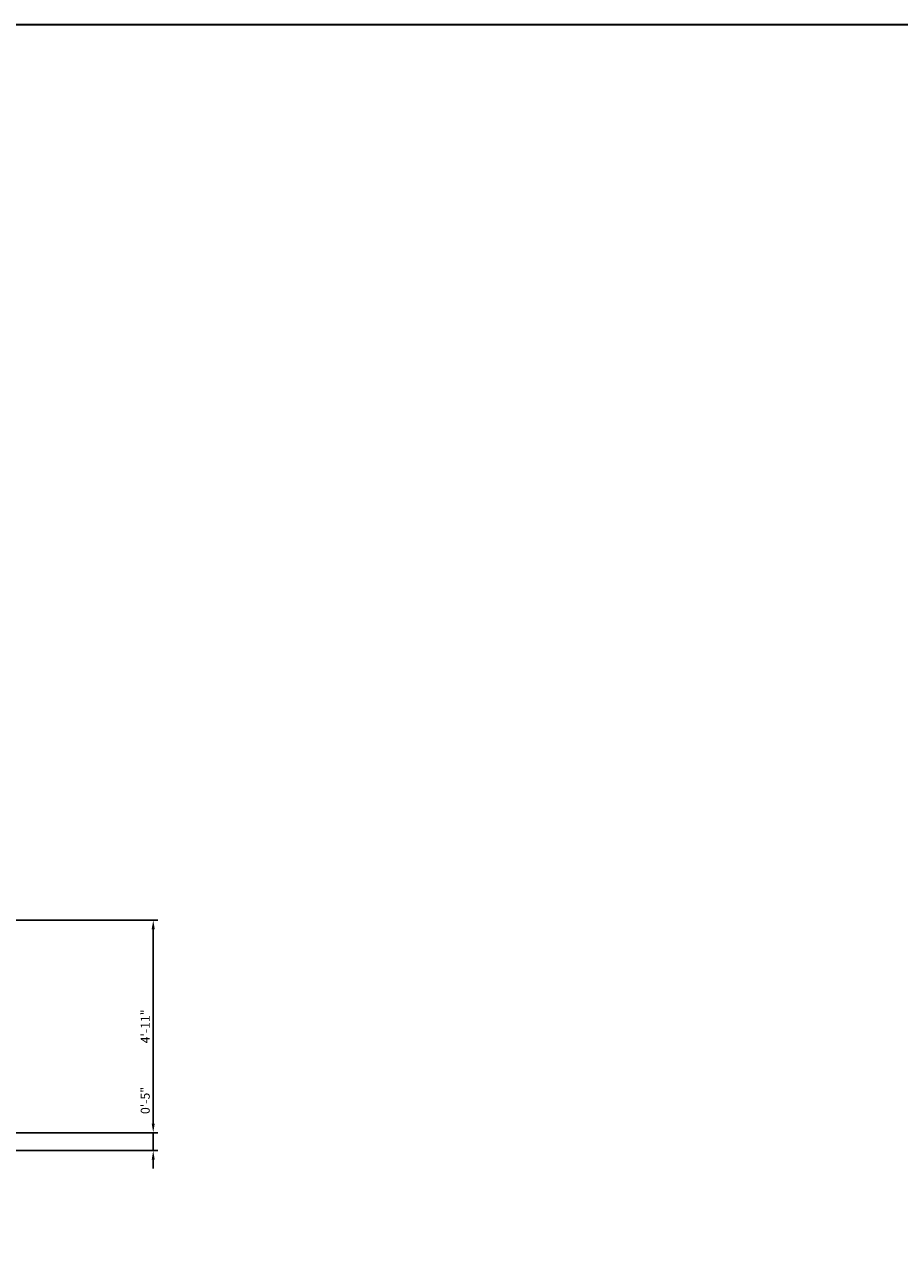
# Model space of a CAD drawing. Units: inches. Extents: x 2020 to 7901, y 1581 to 3943.
# Tile 17 of 17: x 3294 to 3537, y 2728 to 3067. Entities that reach past the tile are written whole.
import ezdxf

# ---------------------------------------------------------------- set-up
doc = ezdxf.new("R2010")
doc.units = ezdxf.units.IN
doc.layers.add('A-ANNO-DIMS', color=2, linetype='Continuous', lineweight=18)
doc.layers.add('A-ANNO-TTLB', color=7, linetype='Continuous', lineweight=35)
doc.styles.get("Standard").update_dxf_attribs({"font": 'arial.ttf'})
doc.dimstyles.new('ISO-25', dxfattribs={"dimtxt": 2.5, "dimasz": 2.5, "dimexe": 1.25, "dimexo": 0.625, "dimtad": 1, "dimdec": 1, "dimlunit": 3, "dimtxsty": 'Standard', "dimcen": 2.5, "dimadec": 0, "dimazin": 0, "dimtfac": 1, "dimtdec": 1, "dimtmove": 0, "dimatfit": 3, "dimfxl": 1, "dimarcsym": 0})

# ---------------------------------------------------------------- blocks, each defined once
blk = doc.blocks.new('*D159')
at = {"layer": 'A-ANNO-DIMS', "color": 0, "lineweight": -2, "transparency": 16777216}
for p, q in [((3329.38, 2761.71), (3329.38, 2772.1)), ((3257.93, 2759.21), (3330.63, 2759.21)), ((3329.38, 2754.21), (3329.38, 2759.21)), ((3257.93, 2754.21), (3330.63, 2754.21)), ((3329.38, 2751.71), (3329.38, 2749.21))]:
    blk.add_line(p, q, dxfattribs=at)
at = {"layer": 'A-ANNO-DIMS', "color": 0, "transparency": 16777216}
for points in [[(3328.96, 2761.71), (3329.8, 2761.71), (3329.38, 2759.21)], [(3328.96, 2751.71), (3329.8, 2751.71), (3329.38, 2754.21)]]:
    blk.add_solid(points, dxfattribs=at)
at = {"layer": 'DEFPOINTS', "color": 0, "transparency": 16777216}
for p in [(3257.31, 2759.21), (3329.38, 2759.21), (3257.31, 2754.21)]:
    blk.add_point(p, dxfattribs=at)
at = {"layer": 'A-ANNO-DIMS', "color": 0, "transparency": 16777216, "insert": (3327.48, 2768.16), "char_height": 2.5, "attachment_point": 5, "rotation": 90}
blk.add_mtext('0\'-5"', dxfattribs=at)
blk = doc.blocks.new('*D166')
at = {"layer": 'A-ANNO-DIMS', "color": 0, "lineweight": -2, "transparency": 16777216}
for p, q in [((3174.76, 2818.27), (3330.63, 2818.27)), ((3329.38, 2815.77), (3329.38, 2761.71)), ((3257.93, 2759.21), (3330.63, 2759.21))]:
    blk.add_line(p, q, dxfattribs=at)
at = {"layer": 'A-ANNO-DIMS', "color": 0, "transparency": 16777216}
for points in [[(3328.96, 2815.77), (3329.8, 2815.77), (3329.38, 2818.27)], [(3328.96, 2761.71), (3329.8, 2761.71), (3329.38, 2759.21)]]:
    blk.add_solid(points, dxfattribs=at)
at = {"layer": 'DEFPOINTS', "color": 0, "transparency": 16777216}
for p in [(3174.14, 2818.27), (3257.31, 2759.21), (3329.38, 2759.21)]:
    blk.add_point(p, dxfattribs=at)
at = {"layer": 'A-ANNO-DIMS', "color": 0, "transparency": 16777216, "insert": (3327.5, 2788.74), "char_height": 2.5, "attachment_point": 5, "rotation": 90}
blk.add_mtext('4\'-11"', dxfattribs=at)

msp = doc.modelspace()

# ---------------------------------------------------------------- linework, layer by layer
at = {"layer": 'A-ANNO-TTLB'}
msp.add_lwpolyline([(2019.8, 3067.25), (4199.03, 3067.25), (4199.03, 1580.73), (2019.8, 1580.73)], close=True, dxfattribs=at)

# ---------------------------------------------------------------- dimensions: what is measured, and where the dimension line sits
at = {"layer": 'A-ANNO-DIMS'}
for p1, picture, middle in [((3174.14, 2818.27), '*D166', (3327.5, 2788.74)), ((3257.31, 2754.21), '*D159', (3327.48, 2768.16))]:
    dim = msp.add_linear_dim(base=(3329.38, 2759.21), p1=p1, p2=(3257.31, 2759.21), angle=90, dimstyle='ISO-25', override={"dimdec": 1, "dimlfac": 1, "dimrnd": 0, "dimzin": 1, "dimdsep": 46, "dimlunit": 4, "dimfrac": 2}, dxfattribs=at)
    dim.commit()
    dim.dimension.update_dxf_attribs({"geometry": picture, "text_midpoint": middle})

doc.saveas('drawing.dxf')
